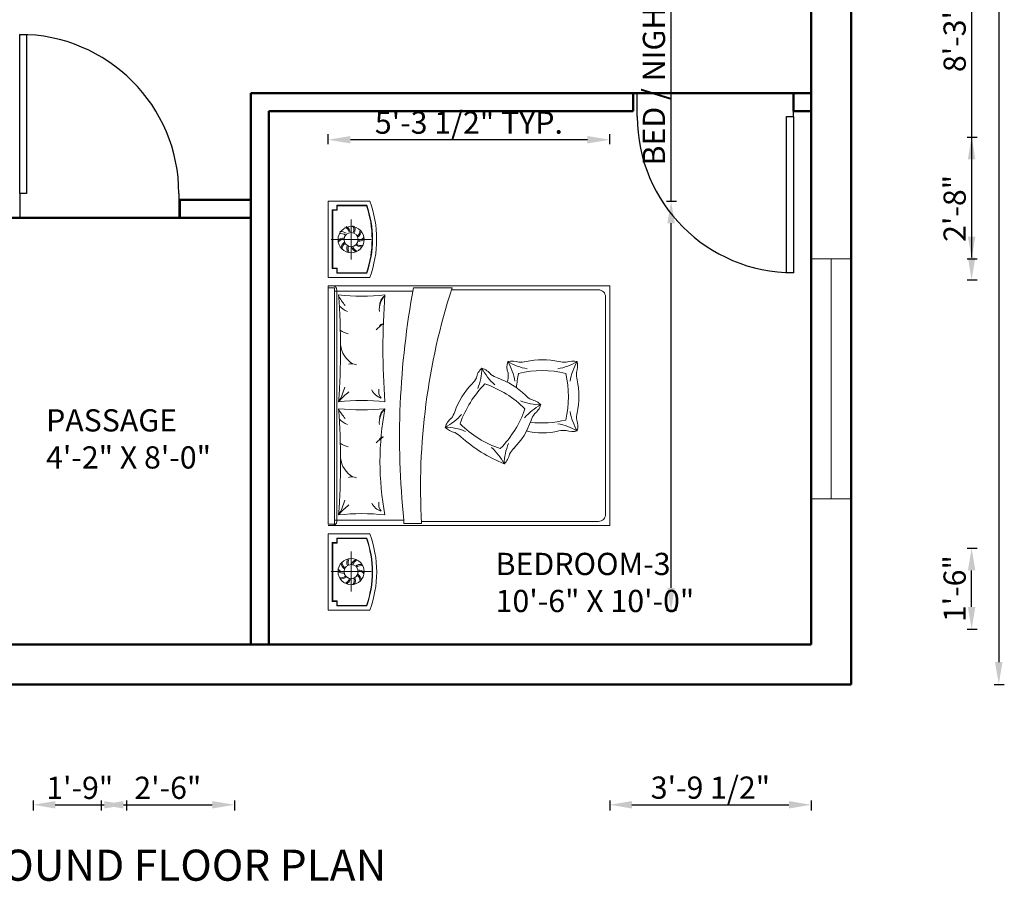
# Model space of a CAD drawing. Units: inches. Extents: x -8 to 396, y -471 to 106.
# Tile 2 of 4: x 167 to 388, y -471 to -277. Entities that reach past the tile are written whole.
import ezdxf

# ---------------------------------------------------------------- set-up
doc = ezdxf.new("R2010")
doc.units = ezdxf.units.IN
for name, color, linetype, lineweight in [('A-ANNO-DIMS', 2, 'Continuous', 18), ('A-ANNO-TEXT', 7, 'Continuous', 25), ('A-AREA-IDEN', 7, 'Continuous', 18), ('A-DOOR', 3, 'Continuous', 25), ('A-GLAZ', 4, 'Continuous', 18), ('A-WALL', 7, 'Continuous', 50), ('furn', 8, 'Continuous', 18)]:
    doc.layers.add(name, color=color, linetype=linetype, lineweight=lineweight)
doc.styles.get("Standard").update_dxf_attribs({"font": 'arial.ttf'})
doc.dimstyles.new('ISO-25', dxfattribs={"dimtxt": 5, "dimasz": 5, "dimexe": 1.25, "dimexo": 0.625, "dimtad": 1, "dimlunit": 3, "dimtxsty": 'Standard', "dimcen": 2.5, "dimadec": 0, "dimazin": 0, "dimtfac": 1, "dimtmove": 0, "dimatfit": 3, "dimfxl": 1, "dimfxlon": 1, "dimarcsym": 0})

# ---------------------------------------------------------------- blocks, each defined once
blk = doc.blocks.new('*U5')
for p, q in [((0, 0), (0, -6)), ((40, 0), (40, -6))]:
    blk.add_line(p, q)
blk.add_lwpolyline([(0, 0), (0, 40), (1.75, 40), (1.75, 0)], close=True)
blk.add_arc((0, 0), 40, 0, 90)
blk = doc.blocks.new('*D9')
at = {"layer": 'A-ANNO-DIMS', "color": 0, "lineweight": -2, "transparency": 16777216}
for p, q in [((386.16, 16.55), (388.41, 16.55)), ((387.16, 11.55), (387.16, -421.87)), ((386.16, -426.87), (388.41, -426.87))]:
    blk.add_line(p, q, dxfattribs=at)
at = {"layer": 'A-ANNO-DIMS', "color": 0, "transparency": 16777216}
for points in [[(386.32, 11.55), (387.99, 11.55), (387.16, 16.55)], [(386.32, -421.87), (387.99, -421.87), (387.16, -426.87)]]:
    blk.add_solid(points, dxfattribs=at)
at = {"layer": 'Defpoints', "color": 0, "transparency": 16777216}
for p in [(353.97, 16.55), (353.97, -426.87), (387.16, -426.87)]:
    blk.add_point(p, dxfattribs=at)
at = {"layer": 'A-ANNO-DIMS', "color": 0, "transparency": 16777216, "insert": (383.98, -205.16), "char_height": 5, "attachment_point": 5, "rotation": 90}
blk.add_mtext('36\'-11.43"', dxfattribs=at)
blk = doc.blocks.new('BED-DOUBLE-WITH-NIGHTSTANDS')
for p, q in [((8.67, 53.66), (8.67, 62.66)), ((83.36, 53.66), (83.36, 62.65)), ((19.97, 61.4), (72.06, 61.4)), ((20.23, 61.87), (20.23, 46.28)), ((71.76, 61.87), (71.76, 44.26)), ((4.17, 58.16), (13.17, 58.16)), ((87.86, 58.16), (78.86, 58.16))]:
    blk.add_line(p, q)
for points in [[(0, 53.96), (0, 63.32), (17.16, 63.32), (17.16, 53.96, -0.181818)], [(92.03, 53.97), (92.03, 63.33), (74.87, 63.33), (74.87, 53.97, 0.181818)], [(21.42, 50.55, 0.058596), (21.42, 60.97, 0.036889), (45.31, 60.97, 0.052163), (45.31, 50.55, 0.093111)], [(46.86, 50.55, 0.058596), (46.86, 60.97, 0.036648), (70.91, 60.97, 0.052163), (70.91, 50.55, 0.036967)], [(19.5, 46.28), (20.23, 46.28, -0.072944), (72.49, 44.11), (72.49, 35.45, 0.092568), (19.5, 42.31)]]:
    blk.add_lwpolyline(points, format="xyb", close=True)
for points in [[(1.97, 62.39), (1.97, 61.36), (0.94, 61.36)], [(2.06, 62.39), (2.06, 61.26), (0.94, 61.26)], [(1.97, 62.39), (15.19, 62.39)], [(1.97, 62.29), (15.19, 62.29)], [(15.1, 62.39), (15.1, 61.26), (16.22, 61.26)], [(15.19, 62.39), (15.19, 61.36), (16.22, 61.36)], [(19.03, 63.33), (19.03, 0), (73, 0), (73, 63.33)], [(72.49, 63.33), (72.49, 61.87), (19.34, 61.87), (19.34, 63.33), (73, 63.33)], [(76.84, 62.39), (76.84, 61.36), (75.81, 61.36)], [(76.93, 62.39), (76.93, 61.27), (75.81, 61.27)], [(90.06, 62.39), (76.84, 62.39)], [(90.06, 62.3), (76.84, 62.3)], [(89.97, 62.39), (89.97, 61.27), (91.09, 61.27)], [(90.06, 62.39), (90.06, 61.36), (91.09, 61.36)]]:
    blk.add_lwpolyline(points)
for points in [[(16.22, 61.36), (16.22, 54.62, -0.167087), (0.94, 54.62), (0.94, 61.36)], [(16.13, 61.36), (16.13, 54.68, -0.165559), (1.03, 54.68), (1.03, 61.36)], [(75.81, 61.36), (75.81, 54.62, 0.167087), (91.09, 54.62), (91.09, 61.36)], [(75.9, 61.36), (75.9, 54.69, 0.165559), (91, 54.69), (91, 61.36)], [(19.97, 42.34), (19.97, 2.5, 0.414214), (21.53, 0.94), (70.5, 0.94, 0.414214), (72.06, 2.5), (72.06, 35.61)], [(40.22, 32.4, 0.091296), (41.17, 36.97, 0.091296), (44.05, 33.3, 0.091296)], [(36.36, 24.6, 0.111006), (45.27, 19.06, 0.119549), (50.89, 28.07, 0.107813), (42, 33.64)], [(41.95, 33.62, 0.121865), (36.36, 24.6, 0.121865)], [(49.84, 29.69, 0.091296), (54.41, 28.73, 0.091296), (50.72, 25.86, 0.091296)], [(37.49, 22.77, 0.091296), (32.92, 23.74, 0.091296), (36.61, 26.6, 0.091296)], [(46.16, 15.49, 0.159461), (47.37, 17.63, -0.076283), (48.33, 18.96, 0.115075), (52.24, 25.25, -0.076283), (53.02, 26.7, 0.159461), (54.41, 28.73)], [(51.53, 21.31, 0.091296), (55.91, 22.91, 0.091296), (54.3, 18.53, 0.091296)], [(55.91, 7.31, 0.159461), (55.8, 9.77, -0.076283), (55.91, 11.41, 0.115075), (55.91, 18.81, -0.076283), (55.8, 20.45, 0.159461), (55.91, 22.91)], [(42.77, 9.86, 0.111006), (53.27, 9.87, 0.119549), (53.27, 20.49, 0.033212), (50.04, 20.98)], [(47.11, 20.06, 0.091296), (46.16, 15.49, 0.091296), (43.28, 19.16)], [(44.7, 8.91, 0.091296), (40.31, 7.31, 0.091296), (41.93, 11.69, 0.091296)], [(54.3, 11.69, 0.091296), (55.91, 7.31, 0.091296), (51.53, 8.91)]]:
    blk.add_lwpolyline(points, format="xyb")
for centre, radius in [((8.67, 58.16), 2.94), ((83.36, 58.16), 2.94), ((8.67, 58.16), 1.59), ((83.36, 58.16), 1.59)]:
    blk.add_circle(centre, radius)
for centre, radius, start, end in [((19.97, 62.34), 0.936, 180, 270), ((72.06, 62.34), 0.936, 270, 0), ((8.93, 60.36), 1.89, 172.17, 218.4897), ((8.74, 60.32), 1.44, 160.3002, 220.538), ((10.17, 59.78), 1.89, 136.17, 182.4897), ((10, 59.86), 1.44, 124.3002, 184.538), ((10.84, 58.59), 1.89, 100.17, 146.4897), ((10.75, 58.75), 1.44, 88.3002, 148.538), ((26.97, 69.69), 10.33, 237.5379, 257.5233), ((13.61, 51.22), 12.5, 36.4935, 51.2792), ((34.89, 54.79), 5.78, 96.6849, 148.3182), ((40.74, 58.08), 4.06, 141.8174, 169.8987), ((45.87, 57.5), 4.36, 130.5354, 160.3558), ((48.59, 53.82), 7.86, 114.6457, 134.1585), ((39.05, 51.22), 12.5, 36.4935, 51.2792), ((52.41, 69.69), 10.33, 237.5379, 257.5233), ((60.33, 54.79), 5.78, 96.6849, 148.3182), ((66.18, 58.08), 4.06, 141.8174, 169.8987), ((71.31, 57.5), 4.36, 130.5354, 160.3558), ((74.03, 53.82), 7.86, 114.6457, 134.1585), ((81.28, 58.75), 1.44, 31.462, 91.6998), ((81.19, 58.59), 1.89, 33.5103, 79.83), ((82.03, 59.86), 1.44, 355.462, 55.6998), ((81.86, 59.78), 1.89, 357.5103, 43.83), ((83.28, 60.32), 1.44, 319.462, 19.6998), ((83.31, 60.44), 1.89, 321.5103, 7.83), ((6.64, 58.9), 1.44, 232.3002, 292.538), ((7.58, 60.09), 1.89, 208.17, 254.4897), ((7.46, 59.95), 1.44, 196.3002, 256.538), ((10.68, 57.23), 1.89, 64.17, 110.4897), ((10.7, 57.42), 1.44, 52.3002, 112.538), ((9.88, 56.36), 1.44, 16.3002, 76.538), ((9.75, 56.22), 1.89, 28.17, 74.4897), ((27.39, 58.01), 2.59, 335.8927, 16.1192), ((52.83, 58.01), 2.59, 335.8927, 16.1192), ((81.33, 57.42), 1.44, 67.462, 127.6998), ((81.35, 57.23), 1.89, 69.5103, 115.83), ((82.28, 56.22), 1.89, 105.5103, 151.83), ((82.15, 56.36), 1.44, 103.462, 163.6998), ((85.61, 58.98), 1.44, 247.462, 307.6998), ((84.78, 60.03), 1.44, 283.462, 343.6998), ((84.66, 60.17), 1.89, 285.5103, 331.83), ((6.65, 59.08), 1.89, 244.17, 290.4897), ((6.59, 57.56), 1.44, 268.3002, 328.538), ((6.49, 57.72), 1.89, 280.17, 326.4897), ((7.34, 56.45), 1.44, 304.3002, 4.538), ((7.16, 56.53), 1.89, 316.17, 2.4897), ((8.59, 56), 1.44, 340.3002, 40.538), ((8.41, 55.96), 1.89, 352.17, 38.4897), ((83.62, 55.95), 1.89, 141.5103, 187.83), ((83.44, 56), 1.44, 139.462, 199.6998), ((84.86, 56.53), 1.89, 177.5103, 223.83), ((84.69, 56.45), 1.44, 175.462, 235.6998), ((85.53, 57.72), 1.89, 213.5103, 259.83), ((85.44, 57.56), 1.44, 211.462, 271.6998), ((85.59, 59.16), 1.89, 249.5103, 295.83), ((25.53, 50.31), 3.47, 114.2916, 160.9896), ((50.97, 50.31), 3.47, 114.2916, 160.9896), ((23.73, 49.58), 2.37, 76.4823, 128.5563), ((28.45, 43.29), 13.02, 36.2085, 45.0849), ((38.09, 50.99), 0.874, 353.7543, 77.2187), ((42.26, 47.56), 4.26, 44.406, 96.8342), ((43.06, 49.05), 2.7, 33.6349, 90.8456), ((49.17, 49.58), 2.37, 76.4823, 128.5563), ((53.89, 43.29), 13.02, 36.2085, 45.0849), ((63.53, 50.99), 0.874, 353.7543, 77.2187), ((67.7, 47.56), 4.26, 44.406, 96.8342), ((68.5, 49.05), 2.7, 33.6349, 90.8456), ((43.84, 34.06), 3.95, 132.4658, 168.7065), ((40.13, 33.31), 3.82, 37.2937, 74.0973), ((46.4, 39.96), 5.42, 233.2983, 250.7472), ((64.54, 10.81), 34.16, 138.3818, 157.7644), ((35.14, 37.29), 5.42, 315.5854, 333.0343), ((39.41, 19.4), 16.3, 45.1307, 71.3884), ((54.69, 34.83), 5.42, 225.7718, 243.2208), ((51.59, 26.4), 3.65, 39.4726, 79.6505), ((35.83, 26.42), 3.95, 222.6522, 258.8929), ((32.63, 17.7), 5.42, 45.7718, 63.2208), ((48.11, 7.06), 16.3, 77.0576, 78.7033), ((52.92, 28.24), 5.42, 257.6988, 275.1477), ((54.75, 19.45), 3.65, 71.3996, 111.5774), ((47.9, 33.13), 16.3, 225.1307, 251.3884), ((56.19, 15.11), 16.3, 166.8711, 193.1289), ((64.23, 15.22), 22.11, 173.1956, 194.0284), ((40.92, 12.57), 5.42, 53.2983, 70.7472), ((47.68, 19.75), 4.52, 218.7754, 250.3571), ((35.03, 10.24), 5.42, 355.0387, 12.4877), ((44.12, 8.37), 3.95, 159.3666, 195.6073), ((41.36, 11.12), 3.95, 254.5791, 290.8198), ((43.26, 2.03), 5.42, 77.6988, 95.1477), ((48.06, 23.21), 16.3, 257.0576, 283.3153), ((53, 2.06), 5.42, 85.2252, 102.6741), ((54.95, 11.73), 4.52, 250.7023, 282.284)]:
    blk.add_arc(centre, radius, start, end)
blk = doc.blocks.new('WINDOW-54IN')
blk.add_line((4.5, 54), (4.5, 0))
blk.add_lwpolyline([(0, 54), (9, 54), (9, 0), (0, 0)], close=True)
blk = doc.blocks.new('*D16')
at = {"layer": 'A-ANNO-DIMS', "color": 0, "lineweight": -2, "transparency": 16777216}
for p, q in [((313.46, -318.14), (313.46, -209.45)), ((312.46, -318.14), (314.71, -318.14)), ((313.46, -405.17), (313.46, -323.14)), ((312.46, -410.17), (314.71, -410.17))]:
    blk.add_line(p, q, dxfattribs=at)
at = {"layer": 'A-ANNO-DIMS', "color": 0, "transparency": 16777216}
for points in [[(312.63, -323.14), (314.3, -323.14), (313.46, -318.14)], [(312.63, -405.17), (314.3, -405.17), (313.46, -410.17)]]:
    blk.add_solid(points, dxfattribs=at)
at = {"layer": 'Defpoints', "color": 0, "transparency": 16777216}
for p in [(299.66, -318.14), (313.46, -318.14), (299.66, -410.17)]:
    blk.add_point(p, dxfattribs=at)
at = {"layer": 'A-ANNO-DIMS', "color": 0, "transparency": 16777216, "insert": (310.25, -261.3), "char_height": 5, "attachment_point": 5, "rotation": 90}
blk.add_mtext('BED / NIGHTSTANDS 7\'-8" TYP.', dxfattribs=at)
blk = doc.blocks.new('*D17')
at = {"layer": 'A-ANNO-DIMS', "color": 0, "lineweight": -2, "transparency": 16777216}
for p, q in [((236.33, -305.34), (236.33, -303.09)), ((299.66, -305.34), (299.66, -303.09)), ((294.66, -304.34), (241.33, -304.34))]:
    blk.add_line(p, q, dxfattribs=at)
at = {"layer": 'A-ANNO-DIMS', "color": 0, "transparency": 16777216}
for points in [[(241.33, -303.5), (241.33, -305.17), (236.33, -304.34)], [(294.66, -303.5), (294.66, -305.17), (299.66, -304.34)]]:
    blk.add_solid(points, dxfattribs=at)
at = {"layer": 'Defpoints', "color": 0, "transparency": 16777216}
for p in [(236.33, -304.34), (236.33, -318.14), (299.66, -318.14)]:
    blk.add_point(p, dxfattribs=at)
at = {"layer": 'A-ANNO-DIMS', "color": 0, "transparency": 16777216, "insert": (267.99, -301.13), "char_height": 5, "attachment_point": 5}
blk.add_mtext('5\'-3 1/2" TYP.', dxfattribs=at)
blk = doc.blocks.new('*D33')
at = {"layer": 'A-ANNO-DIMS', "color": 0, "lineweight": -2, "transparency": 16777216}
for p, q in [((380.06, -232.04), (382.31, -232.04)), ((381.06, -237.04), (381.06, -326.13)), ((380.06, -331.13), (382.31, -331.13))]:
    blk.add_line(p, q, dxfattribs=at)
at = {"layer": 'A-ANNO-DIMS', "color": 0, "transparency": 16777216}
for points in [[(380.22, -237.04), (381.89, -237.04), (381.06, -232.04)], [(380.22, -326.13), (381.89, -326.13), (381.06, -331.13)]]:
    blk.add_solid(points, dxfattribs=at)
at = {"layer": 'Defpoints', "color": 0, "transparency": 16777216}
for p in [(353.97, -232.04), (353.97, -331.13), (381.06, -331.13)]:
    blk.add_point(p, dxfattribs=at)
at = {"layer": 'A-ANNO-DIMS', "color": 0, "transparency": 16777216, "insert": (377.88, -281.58), "char_height": 5, "attachment_point": 5, "rotation": 90}
blk.add_mtext('8\'-3"', dxfattribs=at)
blk = doc.blocks.new('*D42')
at = {"layer": 'A-ANNO-DIMS', "color": 0, "lineweight": -2, "transparency": 16777216}
for p, q in [((380.06, -303.72), (382.31, -303.72)), ((381.06, -308.72), (381.06, -330.84)), ((380.06, -335.84), (382.31, -335.84))]:
    blk.add_line(p, q, dxfattribs=at)
at = {"layer": 'A-ANNO-DIMS', "color": 0, "transparency": 16777216}
for points in [[(380.22, -308.72), (381.89, -308.72), (381.06, -303.72)], [(380.22, -330.84), (381.89, -330.84), (381.06, -335.84)]]:
    blk.add_solid(points, dxfattribs=at)
at = {"layer": 'Defpoints', "color": 0, "transparency": 16777216}
for p in [(62.97, -303.72), (60.39, -335.84), (381.06, -335.84)]:
    blk.add_point(p, dxfattribs=at)
at = {"layer": 'A-ANNO-DIMS', "color": 0, "transparency": 16777216, "insert": (377.88, -319.78), "char_height": 5, "attachment_point": 5, "rotation": 90}
blk.add_mtext('2\'-8"', dxfattribs=at)
blk = doc.blocks.new('*D44')
at = {"layer": 'A-ANNO-DIMS', "color": 0, "lineweight": -2, "transparency": 16777216}
for p, q in [((380.06, -396.22), (382.31, -396.22)), ((381.06, -409.44), (381.06, -401.22)), ((380.06, -414.44), (382.31, -414.44))]:
    blk.add_line(p, q, dxfattribs=at)
at = {"layer": 'A-ANNO-DIMS', "color": 0, "transparency": 16777216}
for points in [[(380.22, -401.22), (381.89, -401.22), (381.06, -396.22)], [(380.22, -409.44), (381.89, -409.44), (381.06, -414.44)]]:
    blk.add_solid(points, dxfattribs=at)
at = {"layer": 'Defpoints', "color": 0, "transparency": 16777216}
for p in [(110.29, -396.22), (381.06, -396.22), (110.29, -414.44)]:
    blk.add_point(p, dxfattribs=at)
at = {"layer": 'A-ANNO-DIMS', "color": 0, "transparency": 16777216, "insert": (377.88, -405.33), "char_height": 5, "attachment_point": 5, "rotation": 90}
blk.add_mtext('1\'-6"', dxfattribs=at)
blk = doc.blocks.new('*D45')
at = {"layer": 'A-ANNO-DIMS', "color": 0, "lineweight": -2, "transparency": 16777216}
for p, q in [((299.66, -452.96), (299.66, -455.21)), ((344.97, -452.96), (344.97, -455.21)), ((304.66, -453.96), (339.97, -453.96))]:
    blk.add_line(p, q, dxfattribs=at)
at = {"layer": 'A-ANNO-DIMS', "color": 0, "transparency": 16777216}
for points in [[(304.66, -453.13), (304.66, -454.8), (299.66, -453.96)], [(339.97, -453.13), (339.97, -454.8), (344.97, -453.96)]]:
    blk.add_solid(points, dxfattribs=at)
at = {"layer": 'Defpoints', "color": 0, "transparency": 16777216}
for p in [(299.66, -391.14), (344.97, -417.87), (344.97, -453.96)]:
    blk.add_point(p, dxfattribs=at)
at = {"layer": 'A-ANNO-DIMS', "color": 0, "transparency": 16777216, "insert": (322.31, -450.75), "char_height": 5, "attachment_point": 5}
blk.add_mtext('3\'-9 1/2"', dxfattribs=at)
blk = doc.blocks.new('*D46')
at = {"layer": 'A-ANNO-DIMS', "color": 0, "lineweight": -2, "transparency": 16777216}
for p, q in [((185.28, -452.96), (185.28, -455.21)), ((215.28, -452.96), (215.28, -455.21)), ((190.28, -453.96), (210.28, -453.96))]:
    blk.add_line(p, q, dxfattribs=at)
at = {"layer": 'A-ANNO-DIMS', "color": 0, "transparency": 16777216}
for points in [[(190.28, -453.13), (190.28, -454.8), (185.28, -453.96)], [(210.28, -453.13), (210.28, -454.8), (215.28, -453.96)]]:
    blk.add_solid(points, dxfattribs=at)
at = {"layer": 'Defpoints', "color": 0, "transparency": 16777216}
for p in [(185.28, -87.87), (215.28, -87.87), (215.28, -453.96)]:
    blk.add_point(p, dxfattribs=at)
at = {"layer": 'A-ANNO-DIMS', "color": 0, "transparency": 16777216, "insert": (200.28, -450.79), "char_height": 5, "attachment_point": 5}
blk.add_mtext('2\'-6"', dxfattribs=at)
blk = doc.blocks.new('*D48')
at = {"layer": 'A-ANNO-DIMS', "color": 0, "lineweight": -2, "transparency": 16777216}
for p, q in [((169.97, -452.96), (169.97, -455.21)), ((190.97, -452.96), (190.97, -455.21)), ((174.97, -453.96), (185.97, -453.96))]:
    blk.add_line(p, q, dxfattribs=at)
at = {"layer": 'A-ANNO-DIMS', "color": 0, "transparency": 16777216}
for points in [[(174.97, -453.13), (174.97, -454.8), (169.97, -453.96)], [(185.97, -453.13), (185.97, -454.8), (190.97, -453.96)]]:
    blk.add_solid(points, dxfattribs=at)
at = {"layer": 'Defpoints', "color": 0, "transparency": 16777216}
for p in [(169.97, 0.13), (190.97, 0.13), (190.97, -453.96)]:
    blk.add_point(p, dxfattribs=at)
at = {"layer": 'A-ANNO-DIMS', "color": 0, "transparency": 16777216, "insert": (180.47, -450.79), "char_height": 5, "attachment_point": 5}
blk.add_mtext('1\'-9"', dxfattribs=at)
blk = doc.blocks.new('*D50')
at = {"layer": 'A-ANNO-DIMS', "color": 0, "lineweight": -2, "transparency": 16777216}
for p, q in [((166.97, 94.22), (166.97, 96.47)), ((202.97, 94.22), (202.97, 96.47)), ((171.97, 95.22), (197.97, 95.22))]:
    blk.add_line(p, q, dxfattribs=at)
at = {"layer": 'A-ANNO-DIMS', "color": 0, "transparency": 16777216}
for points in [[(171.97, 96.05), (171.97, 94.38), (166.97, 95.22)], [(197.97, 96.05), (197.97, 94.38), (202.97, 95.22)]]:
    blk.add_solid(points, dxfattribs=at)
at = {"layer": 'Defpoints', "color": 0, "transparency": 16777216}
for p in [(202.97, 95.22), (166.97, -317.87), (202.97, -317.87)]:
    blk.add_point(p, dxfattribs=at)
at = {"layer": 'A-ANNO-DIMS', "color": 0, "transparency": 16777216, "insert": (184.97, 98.4), "char_height": 5, "attachment_point": 5}
blk.add_mtext('3\'-0"', dxfattribs=at)
blk = doc.blocks.new('*D52')
at = {"layer": 'A-ANNO-DIMS', "color": 0, "lineweight": -2, "transparency": 16777216}
for p, q in [((304.97, 94.22), (304.97, 96.47)), ((340.97, 94.22), (340.97, 96.47)), ((309.97, 95.22), (335.97, 95.22))]:
    blk.add_line(p, q, dxfattribs=at)
at = {"layer": 'A-ANNO-DIMS', "color": 0, "transparency": 16777216}
for points in [[(309.97, 96.05), (309.97, 94.38), (304.97, 95.22)], [(335.97, 96.05), (335.97, 94.38), (340.97, 95.22)]]:
    blk.add_solid(points, dxfattribs=at)
at = {"layer": 'Defpoints', "color": 0, "transparency": 16777216}
for p in [(340.97, 95.22), (304.97, -293.87), (340.97, -293.87)]:
    blk.add_point(p, dxfattribs=at)
at = {"layer": 'A-ANNO-DIMS', "color": 0, "transparency": 16777216, "insert": (322.97, 98.4), "char_height": 5, "attachment_point": 5}
blk.add_mtext('3\'-0"', dxfattribs=at)

msp = doc.modelspace()

# ---------------------------------------------------------------- linework, layer by layer
at = {"layer": 'A-WALL'}
for p, q in [((353.966, 17.126), (353.966, -426.874)), ((344.966, 8.126), (344.966, -417.874)), ((218.966, -417.874), (218.966, -293.874)), ((222.966, -293.874), (218.966, -293.874)), ((344.966, -293.874), (222.966, -293.874)), ((304.966, -293.874), (304.966, -297.874)), ((340.966, -293.874), (340.966, -297.874)), ((222.966, -417.874), (222.966, -297.874)), ((304.966, -297.874), (222.966, -297.874)), ((344.966, -297.874), (340.966, -297.874)), ((218.966, -317.874), (202.966, -317.874)), ((202.966, -317.874), (202.966, -321.874)), ((218.966, -321.874), (162.966, -321.874)), ((218.966, -417.874), (162.966, -417.874)), ((222.966, -417.874), (218.966, -417.874)), ((344.966, -417.874), (222.966, -417.874)), ((353.966, -426.874), (29.966, -426.874))]:
    msp.add_line(p, q, dxfattribs=at)

# ---------------------------------------------------------------- block references
at = {"layer": 'A-DOOR', "xscale": 0.894851635990925, "yscale": 0.894851635990925, "zscale": 0.894851635990925}
msp.add_blockref('*U5', (166.966, -316.451), dxfattribs=at)
at = {"layer": 'A-DOOR', "xscale": 0.8776804145844607, "yscale": 0.8776804145844607, "zscale": 0.8776804145844607, "rotation": 180}
msp.add_blockref('*U5', (340.966, -299.14), dxfattribs=at)
at = {"layer": 'A-GLAZ'}
msp.add_blockref('WINDOW-54IN', (344.966, -385.125), dxfattribs=at)
at = {"layer": 'furn', "rotation": 90.00000000000011}
msp.add_blockref('BED-DOUBLE-WITH-NIGHTSTANDS', (299.658, -410.169), dxfattribs=at)

# ---------------------------------------------------------------- texts
at = {"layer": 'A-ANNO-TEXT', "insert": (150.401, -464.054), "char_height": 7, "attachment_point": 1}
msp.add_mtext_dynamic_manual_height_columns('GROUND FLOOR PLAN', width=215.36302, gutter_width=12.5, heights=[0], dxfattribs=at)
at = {"layer": 'A-AREA-IDEN', "char_height": 5, "attachment_point": 1}
for s, width, insert in [('PASSAGE\\P4\'-2" X 8\'-0"', 50.55687, (172.898, -364.974)), ('BEDROOM-3\\P10\'-6" X 10\'-0"', 45.1134, (274.004, -397.274))]:
    msp.add_mtext_dynamic_manual_height_columns(s, width=width, gutter_width=12.5, heights=[0], dxfattribs=dict(at, insert=insert))

# ---------------------------------------------------------------- dimensions: what is measured, and where the dimension line sits
at = {"layer": 'A-ANNO-DIMS'}
for base, p1, p2, picture, middle in [((202.966, 95.216), (166.966, -317.874), (202.966, -317.874), '*D50', (184.966, 98.396)), ((340.966, 95.216), (304.966, -293.874), (340.966, -293.874), '*D52', (322.966, 98.396)), ((190.966, -453.964), (169.966, 0.126), (190.966, 0.126), '*D48', (180.466, -450.786)), ((215.282, -453.964), (185.282, -87.874), (215.282, -87.874), '*D46', (200.282, -450.786)), ((344.966, -453.964), (299.658, -391.14), (344.966, -417.874), '*D45', (322.312, -450.752))]:
    dim = msp.add_linear_dim(base=base, p1=p1, p2=p2, dimstyle='ISO-25', override={"dimdec": 1, "dimlfac": 1, "dimrnd": 0, "dimzin": 1, "dimdsep": 46, "dimlunit": 4, "dimfrac": 2}, dxfattribs=at)
    dim.commit()
    dim.dimension.update_dxf_attribs({"geometry": picture, "text_midpoint": middle})
for base, p1, p2, override, picture, middle in [((387.1551, -426.874), (353.9656, 16.5511), (353.9656, -426.874), {"dimclrd": 0, "dimclre": 0, "dimclrt": 0}, '*D9', (383.9755, -205.1614)), ((381.056, -331.125), (353.966, -232.037), (353.966, -331.125), {"dimdec": 1, "dimlfac": 1, "dimrnd": 0, "dimzin": 1, "dimdsep": 46, "dimlunit": 4, "dimfrac": 2}, '*D33', (377.876, -281.581)), ((381.056, -335.844), (62.966, -303.723), (60.393, -335.844), {"dimdec": 1, "dimlfac": 1, "dimrnd": 0, "dimzin": 1, "dimdsep": 46, "dimlunit": 4, "dimfrac": 2}, '*D42', (377.878, -319.783)), ((381.056, -396.223), (110.289, -414.441), (110.289, -396.223), {"dimdec": 1, "dimlfac": 1, "dimrnd": 0, "dimzin": 1, "dimdsep": 46, "dimlunit": 4, "dimfrac": 2}, '*D44', (377.878, -405.332))]:
    dim = msp.add_linear_dim(base=base, p1=p1, p2=p2, angle=90, dimstyle='ISO-25', override=override, dxfattribs=at)
    dim.commit()
    dim.dimension.update_dxf_attribs({"geometry": picture, "text_midpoint": middle})
for base, p1, p2, angle, text, picture, middle in [((313.462, -318.141), (299.658, -410.169), (299.658, -318.141), 90, 'BED / NIGHTSTANDS <> TYP.', '*D16', (310.252, -261.295)), ((236.331, -304.337), (299.658, -318.141), (236.331, -318.141), 180, '<> TYP.', '*D17', (267.994, -301.125))]:
    dim = msp.add_linear_dim(base=base, p1=p1, p2=p2, angle=angle, text=text, dimstyle='ISO-25', override={"dimdec": 1, "dimlfac": 1, "dimrnd": 0, "dimzin": 1, "dimdsep": 46, "dimlunit": 4, "dimfrac": 2}, dxfattribs=at)
    dim.commit()
    dim.dimension.update_dxf_attribs({"geometry": picture, "text_midpoint": middle})

doc.saveas('drawing.dxf')
